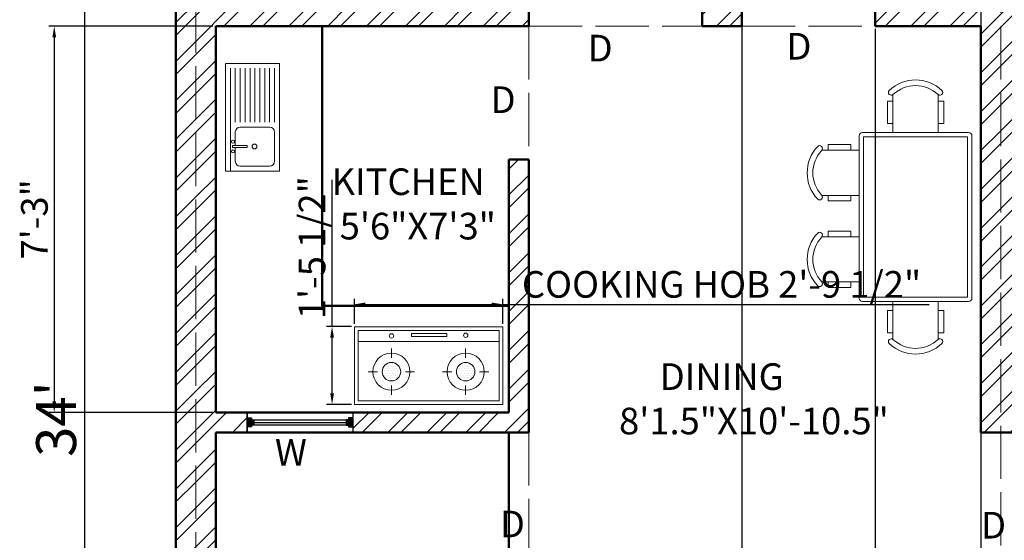
# Model space of a CAD drawing. Units: millimetres. Extents: x 4237 to 5109, y 21391 to 22486.
# Tile 7 of 17: x 4237 to 4458, y 22209 to 22327. Entities that reach past the tile are written whole.
import ezdxf

# ---------------------------------------------------------------- set-up
doc = ezdxf.new("R2010")
doc.units = ezdxf.units.MM
doc.linetypes.add('ACAD_ISO02W100', pattern=[15, 12, -3])
for name, color, linetype, lineweight in [('A-ANNO-DIMS', 2, 'Continuous', 18), ('A-ANNO-TEXT', 7, 'Continuous', 18), ('A-AREA-IDEN', 3, 'Continuous', 18), ('A-FLOR-OVHD', 1, 'ACAD_ISO02W100', 18), ('A-FURN', 8, 'Continuous', 18), ('A-WALL', 7, 'Continuous', 50), ('A-WALL-PATT', 252, 'Continuous', 13), ('windows', 140, 'Continuous', 25)]:
    doc.layers.add(name, color=color, linetype=linetype, lineweight=lineweight)
doc.styles.get("Standard").update_dxf_attribs({"font": 'arial.ttf'})
doc.dimstyles.new('ISO-25', dxfattribs={"dimtxt": 6, "dimasz": 2.5, "dimexe": 1.25, "dimexo": 0.625, "dimtad": 1, "dimdec": 1, "dimlunit": 4, "dimtxsty": 'Standard', "dimcen": 2.5, "dimadec": 0, "dimazin": 0, "dimtfac": 1, "dimtdec": 1, "dimtmove": 0, "dimatfit": 3, "dimfxl": 1, "dimarcsym": 0})

# ---------------------------------------------------------------- blocks, each defined once
blk = doc.blocks.new('A$C678C741B')
for p, q in [((720, 378), (0, 378)), ((0, 0), (0, 378)), ((702, 360), (18, 360)), ((18, 18), (18, 360)), ((277, 329.9), (277, 344.2)), ((277, 344.2), (448.4, 344.2)), ((448.4, 344.2), (448.4, 329.9)), ((702, 18), (702, 360)), ((720, 0), (720, 378)), ((702, 306), (18, 306)), ((448.4, 329.9), (277, 329.9)), ((180, 226.9), (180, 271.9)), ((540, 226.9), (540, 271.9)), ((161.1, 197.3), (161.1, 197.3)), ((172.3, 197.3), (172.3, 197.3)), ((183.6, 197.3), (183.6, 197.3)), ((194.8, 197.3), (194.8, 197.3)), ((521.1, 197.3), (521.1, 197.3)), ((532.3, 197.3), (532.3, 197.3)), ((543.6, 197.3), (543.6, 197.3)), ((554.8, 197.3), (554.8, 197.3)), ((112.5, 159.4), (67.5, 159.4)), ((138.6, 174.8), (138.6, 174.8)), ((138.6, 152.3), (138.6, 152.3)), ((144.2, 186.1), (144.2, 186.1)), ((144.2, 163.6), (144.2, 163.6)), ((149.8, 174.8), (149.8, 174.8)), ((149.8, 152.3), (149.8, 152.3)), ((155.5, 186.1), (155.5, 186.1)), ((155.5, 163.6), (155.5, 163.6)), ((161.1, 174.8), (161.1, 174.8)), ((161.1, 152.3), (161.1, 152.3)), ((166.7, 186.1), (166.7, 186.1)), ((166.7, 163.6), (166.7, 163.6)), ((172.3, 174.8), (172.3, 174.8)), ((172.3, 152.3), (172.3, 152.3)), ((178, 186.1), (178, 186.1)), ((178, 163.6), (178, 163.6)), ((183.6, 174.8), (183.6, 174.8)), ((183.6, 152.3), (183.6, 152.3)), ((189.2, 186.1), (189.2, 186.1)), ((189.2, 163.6), (189.2, 163.6)), ((194.8, 174.8), (194.8, 174.8)), ((194.8, 152.3), (194.8, 152.3)), ((200.5, 186.1), (200.5, 186.1)), ((200.5, 163.6), (200.5, 163.6)), ((206.1, 174.8), (206.1, 174.8)), ((206.1, 152.3), (206.1, 152.3)), ((211.7, 186.1), (211.7, 186.1)), ((211.7, 163.6), (211.7, 163.6)), ((217.3, 174.8), (217.3, 174.8)), ((217.3, 152.3), (217.3, 152.3)), ((223, 163.6), (223, 163.6)), ((292.5, 159.4), (247.5, 159.4)), ((472.5, 159.4), (427.5, 159.4)), ((498.6, 174.8), (498.6, 174.8)), ((498.6, 152.3), (498.6, 152.3)), ((504.2, 186.1), (504.2, 186.1)), ((504.2, 163.6), (504.2, 163.6)), ((509.8, 174.8), (509.8, 174.8)), ((509.8, 152.3), (509.8, 152.3)), ((515.5, 186.1), (515.5, 186.1)), ((515.5, 163.6), (515.5, 163.6)), ((521.1, 174.8), (521.1, 174.8)), ((521.1, 152.3), (521.1, 152.3)), ((526.7, 186.1), (526.7, 186.1)), ((526.7, 163.6), (526.7, 163.6)), ((532.3, 174.8), (532.3, 174.8)), ((532.3, 152.3), (532.3, 152.3)), ((538, 186.1), (538, 186.1)), ((538, 163.6), (538, 163.6)), ((543.6, 174.8), (543.6, 174.8)), ((543.6, 152.3), (543.6, 152.3)), ((549.2, 186.1), (549.2, 186.1)), ((549.2, 163.6), (549.2, 163.6)), ((554.8, 174.8), (554.8, 174.8)), ((554.8, 152.3), (554.8, 152.3)), ((560.5, 186.1), (560.5, 186.1)), ((560.5, 163.6), (560.5, 163.6)), ((566.1, 174.8), (566.1, 174.8)), ((566.1, 152.3), (566.1, 152.3)), ((571.7, 186.1), (571.7, 186.1)), ((571.7, 163.6), (571.7, 163.6)), ((577.3, 174.8), (577.3, 174.8)), ((577.3, 152.3), (577.3, 152.3)), ((583, 163.6), (583, 163.6)), ((652.5, 159.4), (607.5, 159.4)), ((144.2, 141.1), (144.2, 141.1)), ((149.8, 129.8), (149.8, 129.8)), ((155.5, 141.1), (155.5, 141.1)), ((161.1, 129.8), (161.1, 129.8)), ((166.7, 141.1), (166.7, 141.1)), ((166.7, 118.6), (166.7, 118.6)), ((172.3, 129.8), (172.3, 129.8)), ((178, 141.1), (178, 141.1)), ((178, 118.6), (178, 118.6)), ((183.6, 129.8), (183.6, 129.8)), ((189.2, 141.1), (189.2, 141.1)), ((189.2, 118.6), (189.2, 118.6)), ((194.8, 129.8), (194.8, 129.8)), ((200.5, 141.1), (200.5, 141.1)), ((206.1, 129.8), (206.1, 129.8)), ((211.7, 141.1), (211.7, 141.1)), ((504.2, 141.1), (504.2, 141.1)), ((509.8, 129.8), (509.8, 129.8)), ((515.5, 141.1), (515.5, 141.1)), ((521.1, 129.8), (521.1, 129.8)), ((526.7, 141.1), (526.7, 141.1)), ((526.7, 118.6), (526.7, 118.6)), ((532.3, 129.8), (532.3, 129.8)), ((538, 141.1), (538, 141.1)), ((538, 118.6), (538, 118.6)), ((543.6, 129.8), (543.6, 129.8)), ((549.2, 141.1), (549.2, 141.1)), ((549.2, 118.6), (549.2, 118.6)), ((554.8, 129.8), (554.8, 129.8)), ((560.5, 141.1), (560.5, 141.1)), ((566.1, 129.8), (566.1, 129.8)), ((571.7, 141.1), (571.7, 141.1)), ((180, 46.9), (180, 91.9)), ((540, 46.9), (540, 91.9)), ((720, 0), (0, 0)), ((702, 18), (18, 18))]:
    blk.add_line(p, q)
for centre, radius in [((180.2, 333.1), 10.8), ((540.5, 336.3), 10.8), ((180, 159.4), 90), ((540, 159.4), 90), ((180, 159.4), 45), ((540, 159.4), 45)]:
    blk.add_circle(centre, radius)
blk = doc.blocks.new('A$C634174F9')
for p, q in [((0, 0), (0, 550)), ((0, 550), (1100, 550)), ((1100, 550), (1100, 0)), ((0, 500), (1052, 500)), ((100, 450), (240, 450)), ((241, 479), (241, 328)), ((261, 479), (241, 479)), ((261, 479), (261, 328)), ((261, 450), (400, 450)), ((501, 450), (1052, 450)), ((50, 100), (50, 400)), ((241, 328), (261, 328)), ((450, 100), (450, 400)), ((501, 400), (1052, 400)), ((501, 350), (1052, 350)), ((501, 300), (1052, 300)), ((501, 250), (1052, 250)), ((501, 200), (1052, 200)), ((501, 150), (1052, 150)), ((1100, 0), (0, 0)), ((400, 50), (100, 50)), ((1052, 50), (498, 50)), ((501, 100), (1052, 100))]:
    blk.add_line(p, q)
for centre, radius in [((201, 474), 15.3), ((301, 474), 15.3), ((251, 254), 25)]:
    blk.add_circle(centre, radius)
for centre, start, end in [((100, 400), 90, 180), ((100, 400), 90, 180), ((400, 400), 0, 90), ((400, 400), 0, 90), ((100, 100), 180, 270), ((400, 100), 270, 0)]:
    blk.add_arc(centre, 50, start, end)
blk = doc.blocks.new('table dinning')
for p, q in [((4388.77, 22273.66), (4388.77, 22265.14)), ((4398.93, 22265.14), (4398.93, 22273.66)), ((4388.77, 22272.2), (4387.5, 22272.2)), ((4387.5, 22267.12), (4387.5, 22272.2)), ((4398.93, 22272.2), (4400.2, 22272.2)), ((4400.2, 22267.12), (4400.2, 22272.2)), ((4388.77, 22267.12), (4387.5, 22267.12)), ((4398.93, 22267.12), (4400.2, 22267.12)), ((4372.74, 22261.13), (4381.15, 22261.13)), ((4374.21, 22261.13), (4374.21, 22262.4)), ((4379.29, 22262.4), (4374.21, 22262.4)), ((4379.29, 22261.13), (4379.29, 22262.4)), ((4381.15, 22250.97), (4372.74, 22250.97)), ((4374.21, 22250.97), (4374.21, 22249.7)), ((4379.29, 22249.7), (4374.21, 22249.7)), ((4379.29, 22250.97), (4379.29, 22249.7)), ((4374.21, 22241.61), (4374.21, 22242.88)), ((4379.29, 22242.88), (4374.21, 22242.88)), ((4379.29, 22241.61), (4379.29, 22242.88)), ((4372.74, 22241.61), (4381.15, 22241.61)), ((4381.15, 22231.45), (4372.74, 22231.45)), ((4374.21, 22231.45), (4374.21, 22230.18)), ((4379.29, 22230.18), (4374.21, 22230.18)), ((4379.29, 22231.45), (4379.29, 22230.18)), ((4387.5, 22225.06), (4387.5, 22219.98)), ((4388.77, 22225.06), (4387.5, 22225.06)), ((4388.77, 22218.52), (4388.77, 22227.04)), ((4398.93, 22227.04), (4398.93, 22218.52)), ((4398.93, 22225.06), (4400.2, 22225.06)), ((4400.2, 22225.06), (4400.2, 22219.98)), ((4388.77, 22219.98), (4387.5, 22219.98)), ((4398.93, 22219.98), (4400.2, 22219.98))]:
    blk.add_line(p, q)
blk.add_lwpolyline([(4381.91, 22265.14), (4405.79, 22265.14, -0.414214), (4406.55, 22264.38), (4406.55, 22227.8, -0.414214), (4405.79, 22227.04), (4381.91, 22227.04, -0.414214), (4381.15, 22227.8), (4381.15, 22264.38, -0.414214)], format="xyb", close=True)
blk.add_lwpolyline([(4382.15, 22264.14), (4405.55, 22264.14), (4405.55, 22228.04), (4382.15, 22228.04)], close=True)
for centre, radius, start, end in [((4393.85, 22268.32), 8.64, 46.4394, 133.5606), ((4388.37, 22274.16), 0.637, 138.3417, 308.7795), ((4393.85, 22268.32), 7.37, 46.4394, 133.5606), ((4399.33, 22274.16), 0.637, 231.2205, 41.6583), ((4378.09, 22256.05), 8.64, 136.4394, 223.5606), ((4378.09, 22256.05), 7.37, 136.4394, 223.5606), ((4372.25, 22261.53), 0.637, 321.2205, 131.6583), ((4372.25, 22250.57), 0.637, 228.3417, 38.7795), ((4372.25, 22242.01), 0.637, 321.2205, 131.6583), ((4378.09, 22236.53), 8.64, 136.4394, 223.5606), ((4378.09, 22236.53), 7.37, 136.4394, 223.5606), ((4372.25, 22231.05), 0.637, 228.3417, 38.7795), ((4388.37, 22218.02), 0.637, 51.2205, 221.6583), ((4393.85, 22223.86), 7.37, 226.4394, 313.5606), ((4399.33, 22218.02), 0.637, 318.3417, 128.7795), ((4393.85, 22223.86), 8.64, 226.4394, 313.5606)]:
    blk.add_arc(centre, radius, start, end)
blk = doc.blocks.new('*D58')
at = {"layer": 'A-ANNO-DIMS', "color": 0, "lineweight": -2, "transparency": 16777216}
for p, q in [((4271.03, 22440.7), (4249.86, 22440.7)), ((4251.11, 22438.2), (4251.11, 22035.2)), ((4271.03, 22032.7), (4249.86, 22032.7))]:
    blk.add_line(p, q, dxfattribs=at)
at = {"layer": 'A-ANNO-DIMS', "color": 0, "transparency": 16777216}
for points in [[(4250.69, 22438.2), (4251.53, 22438.2), (4251.11, 22440.7)], [(4250.69, 22035.2), (4251.53, 22035.2), (4251.11, 22032.7)]]:
    blk.add_solid(points, dxfattribs=at)
at = {"layer": 'Defpoints', "color": 0, "transparency": 16777216}
for p in [(4271.65, 22440.7), (4251.11, 22032.7), (4271.65, 22032.7)]:
    blk.add_point(p, dxfattribs=at)
at = {"layer": 'A-ANNO-DIMS', "color": 0, "transparency": 16777216, "insert": (4245.89, 22236.7), "char_height": 9, "attachment_point": 5, "rotation": 90}
blk.add_mtext("34'", dxfattribs=at)
blk = doc.blocks.new('WIN-A')
blk.add_line((0, 4.5), (0, 0))
blk.add_lwpolyline([(0, 4.5), (23.8, 4.5), (23.8, 0), (0, 0)], close=True)
blk = doc.blocks.new('*D84')
at = {"layer": 'A-ANNO-DIMS', "color": 0, "lineweight": -2, "transparency": 16777216}
for p, q in [((4311.87, 22258.14), (4311.87, 22263.78)), ((4314.37, 22262.53), (4342.79, 22262.53)), ((4345.29, 22258.14), (4345.29, 22263.78)), ((4345.29, 22262.53), (4441.3, 22262.53))]:
    blk.add_line(p, q, dxfattribs=at)
at = {"layer": 'A-ANNO-DIMS', "color": 0, "transparency": 16777216}
for points in [[(4314.37, 22262.95), (4314.37, 22262.11), (4311.87, 22262.53)], [(4342.79, 22262.95), (4342.79, 22262.11), (4345.29, 22262.53)]]:
    blk.add_solid(points, dxfattribs=at)
at = {"layer": 'Defpoints', "color": 0, "transparency": 16777216}
for p in [(4345.29, 22262.53), (4311.87, 22257.52), (4345.29, 22257.52)]:
    blk.add_point(p, dxfattribs=at)
at = {"layer": 'A-ANNO-DIMS', "color": 0, "transparency": 16777216, "insert": (4394.55, 22266.26), "char_height": 6, "attachment_point": 5}
blk.add_mtext('COOKING HOB 2\'-9 1/2"', dxfattribs=at)
blk = doc.blocks.new('*D85')
at = {"layer": 'A-ANNO-DIMS', "color": 0, "lineweight": -2, "transparency": 16777216}
for p, q in [((4306.86, 22257.52), (4306.86, 22290.63)), ((4311.25, 22257.52), (4305.61, 22257.52)), ((4306.86, 22242.47), (4306.86, 22255.02)), ((4311.25, 22239.97), (4305.61, 22239.97))]:
    blk.add_line(p, q, dxfattribs=at)
at = {"layer": 'A-ANNO-DIMS', "color": 0, "transparency": 16777216}
for points in [[(4306.44, 22255.02), (4307.28, 22255.02), (4306.86, 22257.52)], [(4306.44, 22242.47), (4307.28, 22242.47), (4306.86, 22239.97)]]:
    blk.add_solid(points, dxfattribs=at)
at = {"layer": 'Defpoints', "color": 0, "transparency": 16777216}
for p in [(4306.86, 22257.52), (4311.87, 22257.52), (4311.87, 22239.97)]:
    blk.add_point(p, dxfattribs=at)
at = {"layer": 'A-ANNO-DIMS', "color": 0, "transparency": 16777216, "insert": (4303.13, 22275.32), "char_height": 6, "attachment_point": 5, "rotation": 90}
blk.add_mtext('1\'-5 1/2"', dxfattribs=at)
blk = doc.blocks.new('*D98')
at = {"layer": 'A-ANNO-DIMS', "color": 0, "lineweight": -2, "transparency": 16777216}
for p, q in [((4280.65, 22233.08), (4280.65, 21960.6)), ((4271.65, 22032.08), (4271.65, 21960.6)), ((4274.15, 21961.85), (4278.15, 21961.85)), ((4280.65, 21961.85), (4300.35, 21961.85))]:
    blk.add_line(p, q, dxfattribs=at)
at = {"layer": 'A-ANNO-DIMS', "color": 0, "transparency": 16777216}
for points in [[(4274.15, 21962.27), (4274.15, 21961.43), (4271.65, 21961.85)], [(4278.15, 21962.27), (4278.15, 21961.43), (4280.65, 21961.85)]]:
    blk.add_solid(points, dxfattribs=at)
at = {"layer": 'Defpoints', "color": 0, "transparency": 16777216}
for p in [(4280.65, 22233.7), (4271.65, 22032.7), (4280.65, 21961.85)]:
    blk.add_point(p, dxfattribs=at)
at = {"layer": 'A-ANNO-DIMS', "color": 0, "transparency": 16777216, "insert": (4291.75, 21965.54), "char_height": 6, "attachment_point": 5}
blk.add_mtext('0\'-9"', dxfattribs=at)
blk = doc.blocks.new('*D99')
at = {"layer": 'A-ANNO-DIMS', "color": 0, "lineweight": -2, "transparency": 16777216}
for p, q in [((4280.65, 22233.08), (4280.65, 21960.6)), ((4346.65, 22233.08), (4346.65, 21960.6)), ((4283.15, 21961.85), (4344.15, 21961.85))]:
    blk.add_line(p, q, dxfattribs=at)
at = {"layer": 'A-ANNO-DIMS', "color": 0, "transparency": 16777216}
for points in [[(4283.15, 21962.27), (4283.15, 21961.43), (4280.65, 21961.85)], [(4344.15, 21962.27), (4344.15, 21961.43), (4346.65, 21961.85)]]:
    blk.add_solid(points, dxfattribs=at)
at = {"layer": 'Defpoints', "color": 0, "transparency": 16777216}
for p in [(4280.65, 22233.7), (4346.65, 22233.7), (4346.65, 21961.85)]:
    blk.add_point(p, dxfattribs=at)
at = {"layer": 'A-ANNO-DIMS', "color": 0, "transparency": 16777216, "insert": (4313.65, 21965.54), "char_height": 6, "attachment_point": 5}
blk.add_mtext('5\'-6"', dxfattribs=at)
blk = doc.blocks.new('*D100')
at = {"layer": 'A-ANNO-DIMS', "color": 0, "lineweight": -2, "transparency": 16777216}
for p, q in [((4346.65, 22233.08), (4346.65, 21960.6)), ((4351.15, 22194.08), (4351.15, 21960.6)), ((4344.15, 21961.85), (4341.65, 21961.85)), ((4346.65, 21961.85), (4351.15, 21961.85)), ((4353.65, 21961.85), (4387.33, 21961.85))]:
    blk.add_line(p, q, dxfattribs=at)
at = {"layer": 'A-ANNO-DIMS', "color": 0, "transparency": 16777216}
for points in [[(4344.15, 21962.27), (4344.15, 21961.43), (4346.65, 21961.85)], [(4353.65, 21962.27), (4353.65, 21961.43), (4351.15, 21961.85)]]:
    blk.add_solid(points, dxfattribs=at)
at = {"layer": 'Defpoints', "color": 0, "transparency": 16777216}
for p in [(4346.65, 22233.7), (4351.15, 22194.7), (4351.15, 21961.85)]:
    blk.add_point(p, dxfattribs=at)
at = {"layer": 'A-ANNO-DIMS', "color": 0, "transparency": 16777216, "insert": (4371.74, 21965.58), "char_height": 6, "attachment_point": 5}
blk.add_mtext('0\'-4 1/2"', dxfattribs=at)
blk = doc.blocks.new('*D102')
at = {"layer": 'A-ANNO-DIMS', "color": 0, "lineweight": -2, "transparency": 16777216}
for p, q in [((4461.95, 22233.08), (4461.95, 21960.6)), ((4452.95, 22185.08), (4452.95, 21960.6)), ((4455.45, 21961.85), (4459.45, 21961.85)), ((4461.95, 21961.85), (4481.65, 21961.85))]:
    blk.add_line(p, q, dxfattribs=at)
at = {"layer": 'A-ANNO-DIMS', "color": 0, "transparency": 16777216}
for points in [[(4455.45, 21962.27), (4455.45, 21961.43), (4452.95, 21961.85)], [(4459.45, 21962.27), (4459.45, 21961.43), (4461.95, 21961.85)]]:
    blk.add_solid(points, dxfattribs=at)
at = {"layer": 'Defpoints', "color": 0, "transparency": 16777216}
for p in [(4461.95, 22233.7), (4452.95, 22185.7), (4461.95, 21961.85)]:
    blk.add_point(p, dxfattribs=at)
at = {"layer": 'A-ANNO-DIMS', "color": 0, "transparency": 16777216, "insert": (4473.05, 21965.54), "char_height": 6, "attachment_point": 5}
blk.add_mtext('0\'-9"', dxfattribs=at)
blk = doc.blocks.new('*D108')
at = {"layer": 'A-ANNO-DIMS', "color": 0, "lineweight": -2, "transparency": 16777216}
for p, q in [((4280.03, 22325.2), (4243.05, 22325.2)), ((4244.3, 22322.7), (4244.3, 22240.7)), ((4280.03, 22238.2), (4243.05, 22238.2))]:
    blk.add_line(p, q, dxfattribs=at)
at = {"layer": 'A-ANNO-DIMS', "color": 0, "transparency": 16777216}
for points in [[(4243.88, 22322.7), (4244.72, 22322.7), (4244.3, 22325.2)], [(4243.88, 22240.7), (4244.72, 22240.7), (4244.3, 22238.2)]]:
    blk.add_solid(points, dxfattribs=at)
at = {"layer": 'Defpoints', "color": 0, "transparency": 16777216}
for p in [(4280.65, 22325.2), (4244.3, 22238.2), (4280.65, 22238.2)]:
    blk.add_point(p, dxfattribs=at)
at = {"layer": 'A-ANNO-DIMS', "color": 0, "transparency": 16777216, "insert": (4240.61, 22281.7), "char_height": 6, "attachment_point": 5, "rotation": 90}
blk.add_mtext('7\'-3"', dxfattribs=at)
blk = doc.blocks.new('*D109')
at = {"layer": 'A-ANNO-DIMS', "color": 0, "lineweight": -2, "transparency": 16777216}
for p, q in [((4351.15, 22325.83), (4351.15, 22469.3)), ((4390.15, 22325.83), (4390.15, 22469.3)), ((4353.65, 22468.05), (4387.65, 22468.05))]:
    blk.add_line(p, q, dxfattribs=at)
at = {"layer": 'A-ANNO-DIMS', "color": 0, "transparency": 16777216}
for points in [[(4353.65, 22468.47), (4353.65, 22467.63), (4351.15, 22468.05)], [(4387.65, 22468.47), (4387.65, 22467.63), (4390.15, 22468.05)]]:
    blk.add_solid(points, dxfattribs=at)
at = {"layer": 'Defpoints', "color": 0, "transparency": 16777216}
for p in [(4390.15, 22468.05), (4351.15, 22325.2), (4390.15, 22325.2)]:
    blk.add_point(p, dxfattribs=at)
at = {"layer": 'A-ANNO-DIMS', "color": 0, "transparency": 16777216, "insert": (4370.65, 22471.74), "char_height": 6, "attachment_point": 5}
blk.add_mtext('3\'-3"', dxfattribs=at)
blk = doc.blocks.new('*D110')
at = {"layer": 'A-ANNO-DIMS', "color": 0, "lineweight": -2, "transparency": 16777216}
for p, q in [((4399.15, 22329.08), (4399.15, 21960.6)), ((4452.95, 22329.08), (4452.95, 21960.6)), ((4401.65, 21961.85), (4450.45, 21961.85))]:
    blk.add_line(p, q, dxfattribs=at)
at = {"layer": 'A-ANNO-DIMS', "color": 0, "transparency": 16777216}
for points in [[(4401.65, 21962.27), (4401.65, 21961.43), (4399.15, 21961.85)], [(4450.45, 21962.27), (4450.45, 21961.43), (4452.95, 21961.85)]]:
    blk.add_solid(points, dxfattribs=at)
at = {"layer": 'Defpoints', "color": 0, "transparency": 16777216}
for p in [(4399.15, 22329.7), (4452.95, 22329.7), (4452.95, 21961.85)]:
    blk.add_point(p, dxfattribs=at)
at = {"layer": 'A-ANNO-DIMS', "color": 0, "transparency": 16777216, "insert": (4426.05, 21965.54), "char_height": 6, "attachment_point": 5}
blk.add_mtext('4\'-6"', dxfattribs=at)
blk = doc.blocks.new('*D111')
at = {"layer": 'A-ANNO-DIMS', "color": 0, "lineweight": -2, "transparency": 16777216}
for p, q in [((4399.15, 22324.58), (4399.15, 21960.6)), ((4429.15, 22324.58), (4429.15, 21960.6)), ((4401.65, 21961.85), (4426.65, 21961.85))]:
    blk.add_line(p, q, dxfattribs=at)
at = {"layer": 'A-ANNO-DIMS', "color": 0, "transparency": 16777216}
for points in [[(4401.65, 21962.27), (4401.65, 21961.43), (4399.15, 21961.85)], [(4426.65, 21962.27), (4426.65, 21961.43), (4429.15, 21961.85)]]:
    blk.add_solid(points, dxfattribs=at)
at = {"layer": 'Defpoints', "color": 0, "transparency": 16777216}
for p in [(4399.15, 22325.2), (4429.15, 22325.2), (4429.15, 21961.85)]:
    blk.add_point(p, dxfattribs=at)
at = {"layer": 'A-ANNO-DIMS', "color": 0, "transparency": 16777216, "insert": (4414.15, 21965.54), "char_height": 6, "attachment_point": 5}
blk.add_mtext('2\'-6"', dxfattribs=at)

msp = doc.modelspace()

# ---------------------------------------------------------------- hatches: boundary and pattern name
at = {"layer": 'A-WALL-PATT'}
h = msp.add_hatch(dxfattribs=at)
h.set_pattern_fill('ANSI32', color=256, scale=0.65)
h.paths.add_polyline_path([(4399.15, 22440.7), (4271.65, 22440.7), (4271.65, 22032.7), (4276.15, 22032.7), (4276.15, 22044.7), (4276.15, 22436.2), (4399.15, 22436.2)])
h.paths.add_polyline_path([(4351.15, 22185.7), (4357.15, 22185.7), (4357.15, 22194.7), (4346.65, 22194.7), (4346.65, 22080.7), (4351.15, 22080.7)], flags=16)
h.paths.add_polyline_path([(4351.15, 22295.2), (4346.65, 22295.2), (4346.65, 22238.2), (4311.53, 22238.2), (4311.53, 22233.7), (4351.15, 22233.7)], flags=16)
h = msp.add_hatch(dxfattribs=at)
h.set_pattern_fill('ANSI32', color=256, scale=0.65)
h.paths.add_polyline_path([(4399.15, 22436.2), (4276.15, 22436.2), (4276.15, 22044.7), (4280.65, 22044.7), (4280.65, 22233.7), (4287.73, 22233.7), (4287.73, 22238.2), (4280.65, 22238.2), (4280.65, 22325.2), (4351.15, 22325.2), (4351.15, 22350.7), (4346.65, 22350.7), (4346.65, 22329.7), (4280.65, 22329.7), (4280.65, 22431.7), (4394.65, 22431.7), (4399.15, 22431.7)], flags=17)
h.paths.add_polyline_path([(4351.15, 22185.7), (4357.15, 22185.7), (4357.15, 22194.7), (4346.65, 22194.7), (4346.65, 22080.7), (4351.15, 22080.7)], flags=16)
h.paths.add_polyline_path([(4351.15, 22295.2), (4346.65, 22295.2), (4346.65, 22238.2), (4311.53, 22238.2), (4311.53, 22233.7), (4351.15, 22233.7)], flags=16)
h = msp.add_hatch(dxfattribs=at)
h.set_pattern_fill('ANSI32', color=256, scale=0.65)
h.paths.add_polyline_path([(4399.15, 22410.7), (4414.15, 22410.7), (4414.15, 22415.2), (4394.65, 22415.2), (4394.65, 22350.7), (4390.15, 22350.7), (4390.15, 22325.2), (4399.15, 22325.2)])
h = msp.add_hatch(dxfattribs=at)
h.set_pattern_fill('ANSI32', color=256, scale=0.65)
h.paths.add_polyline_path([(4457.45, 22415.2), (4437.95, 22415.2), (4437.95, 22410.7), (4452.95, 22410.7), (4452.95, 22329.7), (4429.15, 22329.7), (4429.15, 22325.2), (4452.95, 22325.2), (4452.95, 22233.7), (4457.45, 22233.7)])
h = msp.add_hatch(dxfattribs=at)
h.set_pattern_fill('ANSI32', color=256, scale=0.65)
h.paths.add_polyline_path([(4461.95, 22415.2), (4457.45, 22415.2), (4457.45, 22233.7), (4461.95, 22233.7)])
h = msp.add_hatch(color=256, dxfattribs=at)
h.dxf.hatch_style = 1
h.paths.add_polyline_path([(4289.24, 22236.56), (4288.73, 22236.56), (4288.73, 22236.95), (4287.73, 22236.95), (4287.73, 22234.95), (4288.73, 22234.95), (4288.73, 22235.34), (4289.24, 22235.34)])
h = msp.add_hatch(color=256, dxfattribs=at)
h.dxf.hatch_style = 1
h.paths.add_polyline_path([(4311.53, 22236.95), (4310.53, 22236.95), (4310.53, 22236.56), (4310.01, 22236.56), (4310.01, 22235.34), (4310.53, 22235.34), (4310.53, 22234.95), (4311.53, 22234.95)])

# ---------------------------------------------------------------- linework, layer by layer
at = {"layer": 'A-FLOR-OVHD'}
for p, q in [((4457.45, 22415.2), (4457.45, 22032.7)), ((4351.15, 22325.2), (4351.15, 22295.2)), ((4351.15, 22325.2), (4390.15, 22325.2)), ((4399.15, 22325.2), (4429.15, 22325.2)), ((4351.15, 22233.7), (4351.15, 22194.7))]:
    msp.add_line(p, q, dxfattribs=at)
msp.add_lwpolyline([(4640.45, 22032.7), (4640.45, 22436.2), (4276.15, 22436.2), (4276.15, 22032.7)], dxfattribs=at)
at = {"layer": 'A-WALL'}
for p, q in [((4271.65, 22440.7), (4271.65, 22032.7)), ((4399.15, 22410.7), (4399.15, 22325.2)), ((4351.15, 22350.7), (4351.15, 22325.2)), ((4390.15, 22350.7), (4390.15, 22325.2)), ((4429.15, 22329.7), (4429.15, 22325.2)), ((4280.65, 22325.2), (4280.65, 22238.2)), ((4280.65, 22325.2), (4351.15, 22325.2)), ((4390.15, 22325.2), (4399.15, 22325.2)), ((4429.15, 22325.2), (4452.95, 22325.2)), ((4452.95, 22325.2), (4452.95, 22233.7)), ((4346.65, 22295.2), (4351.15, 22295.2)), ((4346.65, 22295.2), (4346.65, 22238.2)), ((4346.65, 22295.2), (4351.15, 22295.2)), ((4351.15, 22295.2), (4351.15, 22233.7)), ((4280.65, 22238.2), (4346.65, 22238.2)), ((4280.65, 22233.7), (4351.15, 22233.7)), ((4280.65, 22233.7), (4280.65, 22044.7)), ((4346.65, 22194.7), (4346.65, 22233.7)), ((4452.95, 22233.7), (4521.95, 22233.7))]:
    msp.add_line(p, q, dxfattribs=at)
msp.add_lwpolyline([(4304.65, 22325.2), (4304.65, 22262.2), (4346.65, 22262.2)], dxfattribs=at)
at = {"layer": 'windows'}
for p, q in [((4311.53, 22238.2), (4311.53, 22233.7)), ((4289.24, 22236.56), (4310.01, 22236.56)), ((4289.24, 22235.95), (4310.01, 22235.95)), ((4310.01, 22235.34), (4289.24, 22235.34))]:
    msp.add_line(p, q, dxfattribs=at)
for points in [[(4287.73, 22236.95), (4288.73, 22236.95), (4288.73, 22236.56), (4289.24, 22236.56), (4289.24, 22235.34), (4288.73, 22235.34), (4288.73, 22234.95), (4287.73, 22234.95)], [(4311.53, 22236.95), (4310.53, 22236.95), (4310.53, 22236.56), (4310.01, 22236.56), (4310.01, 22235.34), (4310.53, 22235.34), (4310.53, 22234.95), (4311.53, 22234.95)]]:
    msp.add_lwpolyline(points, dxfattribs=at)

# ---------------------------------------------------------------- block references
at = {"layer": 'A-FURN', "xscale": 0.0220671414042477, "yscale": 0.0220671414042477, "zscale": 0.0220671414042477, "rotation": 90}
msp.add_blockref('A$C634174F9', (4295, 22292.56), dxfattribs=at)
at = {"layer": 'A-FURN'}
msp.add_blockref('table dinning', (44.38, 36.13), dxfattribs=at)
at = {"layer": 'A-FURN', "xscale": 0.0464103124886305, "yscale": 0.0464103124886305, "zscale": 0.0464103124886305}
msp.add_blockref('A$C678C741B', (4311.87, 22239.97), dxfattribs=at)
at = {"layer": 'windows'}
msp.add_blockref('WIN-A', (4287.73, 22233.7), dxfattribs=at)

# ---------------------------------------------------------------- texts
at = {"layer": 'A-ANNO-TEXT', "char_height": 6, "attachment_point": 1}
for s, insert in [('    D', (4357.08, 22323.27)), ('    D', (4401.83, 22323.68)), ('    D', (4335.22, 22311.65)), ('    W', (4286.66, 22232.18)), ('    D', (4337.31, 22216.06)), ('    D', (4445.65, 22215.79))]:
    msp.add_mtext_dynamic_manual_height_columns(s, width=21.7253, gutter_width=12.5, heights=[0], dxfattribs=dict(at, insert=insert))
at = {"layer": 'A-AREA-IDEN', "char_height": 6, "attachment_point": 1}
for s, width, insert in [('   KITCHEN\\P    5\'6"X7\'3"', 55.7646, (4301.24, 22293.17)), ('      DINING\\P 8\'1.5"X10\'-10.5"', 72.5927, (4369.64, 22249.26))]:
    msp.add_mtext_dynamic_manual_height_columns(s, width=width, gutter_width=12.5, heights=[0], dxfattribs=dict(at, insert=insert))

# ---------------------------------------------------------------- dimensions: what is measured, and where the dimension line sits
at = {"layer": 'A-ANNO-DIMS'}
for base, p1, p2, picture, middle in [((4390.15, 22468.05), (4351.15, 22325.2), (4390.15, 22325.2), '*D109', (4370.65, 22471.74)), ((4452.95, 21961.85), (4399.15, 22329.7), (4452.95, 22329.7), '*D110', (4426.05, 21965.54)), ((4429.15, 21961.85), (4399.15, 22325.2), (4429.15, 22325.2), '*D111', (4414.15, 21965.54)), ((4280.65, 21961.85), (4271.65, 22032.7), (4280.65, 22233.7), '*D98', (4291.75, 21965.54)), ((4346.65, 21961.85), (4280.65, 22233.7), (4346.65, 22233.7), '*D99', (4313.65, 21965.54)), ((4351.15, 21961.85), (4346.65, 22233.7), (4351.15, 22194.7), '*D100', (4371.74, 21965.58)), ((4461.95, 21961.85), (4452.95, 22185.7), (4461.95, 22233.7), '*D102', (4473.05, 21965.54))]:
    dim = msp.add_linear_dim(base=base, p1=p1, p2=p2, dimstyle='ISO-25', override={"dimdec": 1, "dimlfac": 1, "dimrnd": 0, "dimzin": 1, "dimdsep": 46, "dimlunit": 4, "dimfrac": 2}, dxfattribs=at)
    dim.commit()
    dim.dimension.update_dxf_attribs({"geometry": picture, "text_midpoint": middle})
for base, p1, p2, override, picture, middle in [((4251.11, 22032.7), (4271.65, 22440.7), (4271.65, 22032.7), {"dimtxt": 9, "dimclrd": 0, "dimclre": 0, "dimclrt": 0}, '*D58', (4245.89, 22236.7)), ((4244.3, 22238.2), (4280.65, 22325.2), (4280.65, 22238.2), {"dimdec": 1, "dimlfac": 1, "dimrnd": 0, "dimzin": 1, "dimdsep": 46, "dimlunit": 4, "dimfrac": 2}, '*D108', (4240.61, 22281.7)), ((4306.8588, 22257.5167), (4311.8711, 22239.9736), (4311.8711, 22257.5167), {"dimdec": 1, "dimrnd": 0, "dimzin": 1, "dimlunit": 4, "dimfrac": 2}, '*D85', (4303.1314, 22275.3245))]:
    dim = msp.add_linear_dim(base=base, p1=p1, p2=p2, angle=90, dimstyle='ISO-25', override=override, dxfattribs=at)
    dim.commit()
    dim.dimension.update_dxf_attribs({"geometry": picture, "text_midpoint": middle})
dim = msp.add_linear_dim(base=(4345.29, 22262.53), p1=(4311.87, 22257.52), p2=(4345.29, 22257.52), text='COOKING HOB <>', dimstyle='ISO-25', override={"dimdec": 1, "dimrnd": 0, "dimzin": 1, "dimlunit": 4, "dimfrac": 2}, dxfattribs=at)
dim.commit()
dim.dimension.update_dxf_attribs({"geometry": '*D84', "text_midpoint": (4394.55, 22266.26)})

doc.saveas('drawing.dxf')
